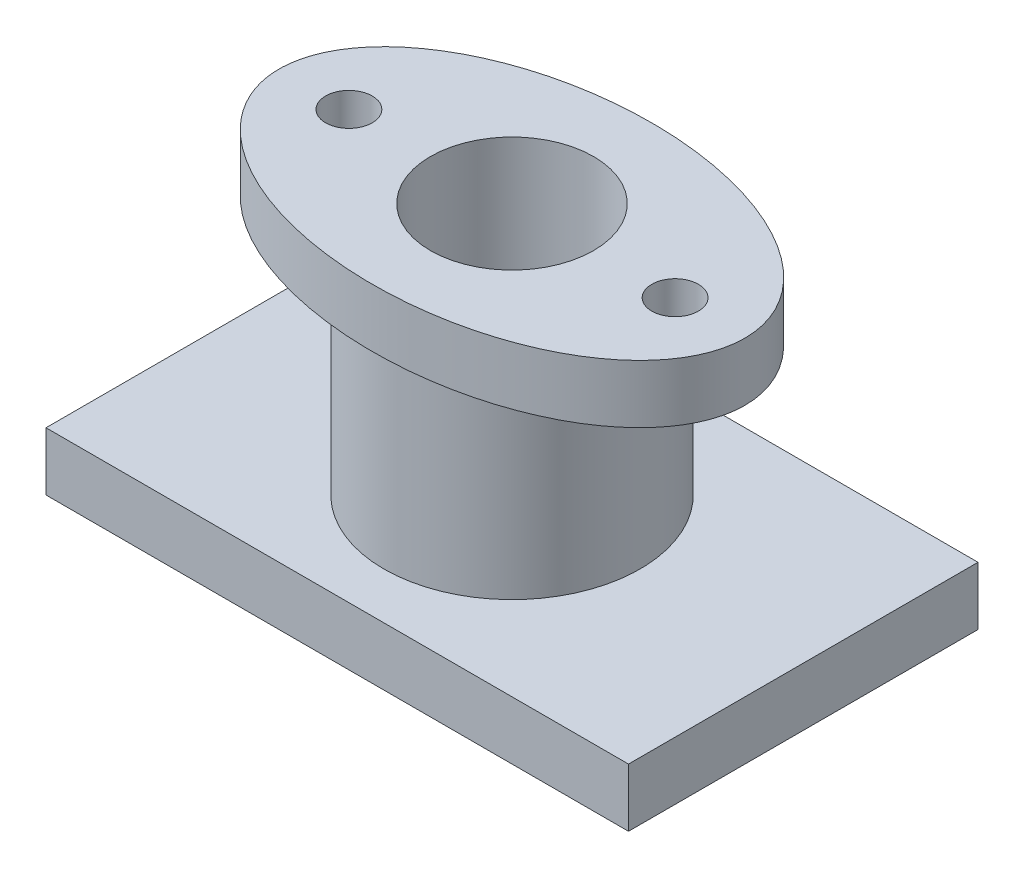
from build123d import *

# Parameters (mm, degrees)
BASE_PLATE_SKETCH_W        = 150
BASE_PLATE_SKETCH_H        = 90
BASE_PLATE_150X90X15_DEPTH = 15
BOSS_TUBE_SKETCH_R         = 33
BOSS_TUBE_SKETCH_R_2       = 21
BOSS_TUBE_66_DEPTH         = 50
OVAL_FLANGE_SKETCH_RX      = 60
OVAL_FLANGE_SKETCH_RY      = 36
OVAL_FLANGE_SKETCH_R       = 21
OVAL_FLANGE_120X72_DEPTH   = 15
BASE_BORE_SKETCH_R         = 16.5
BASE_BORE_33_DEPTH         = 15
FLANGE_BOLT_HOLE_SKETCH_R  = 6
FLANGE_BOLT_HOLE_DEPTH     = 15


with BuildPart() as part:
    # Base Plate Sketch → Base Plate 150x90x15 (new body)
    with BuildSketch(Plane(origin=(0, 0, 0), x_dir=(1, 0, 0), z_dir=(0, 1, 0))):
        Rectangle(BASE_PLATE_SKETCH_W, BASE_PLATE_SKETCH_H)
    extrude(amount=BASE_PLATE_150X90X15_DEPTH)

    # Boss Tube Sketch → Boss Tube Ø66 (add)
    with BuildSketch(Plane(origin=(0, 15, 0), x_dir=(1, 0, 0), z_dir=(0, 1, 0))):
        with Locations(Location((0, 0, 0), (0, 0, 90))):
            Circle(BOSS_TUBE_SKETCH_R)
        with Locations(Location((0, 0, 0), (0, 0, 270))):
            Circle(BOSS_TUBE_SKETCH_R_2, mode=Mode.SUBTRACT)
    extrude(amount=BOSS_TUBE_66_DEPTH)

    # Oval Flange Sketch → Oval Flange 120x72 (add)
    with BuildSketch(Plane(origin=(0, 65, 0), x_dir=(1, 0, 0), z_dir=(0, 1, 0))):
        with Locations((0, 0)):
            Ellipse(OVAL_FLANGE_SKETCH_RX, OVAL_FLANGE_SKETCH_RY)
        with Locations(Location((0, 0, 0), (0, 0, 270))):
            Circle(OVAL_FLANGE_SKETCH_R, mode=Mode.SUBTRACT)
    extrude(amount=OVAL_FLANGE_120X72_DEPTH)

    # Base Bore Sketch → Base Bore Ø33 (cut)
    with BuildSketch(Plane(origin=(0, 15, 0), x_dir=(1, 0, 0), z_dir=(0, 1, 0))):
        with Locations(Location((0, 0, 0), (0, 0, 270))):
            Circle(BASE_BORE_SKETCH_R)
    extrude(amount=-BASE_BORE_33_DEPTH, mode=Mode.SUBTRACT)

    # Flange Bolt Hole Sketch → Flange Bolt Hole (cut)
    with BuildSketch(Plane(origin=(0, 80, 0), x_dir=(1, 0, 0), z_dir=(0, 1, 0))):
        with Locations(Location((-41.995846121, 0, 0), (0, 0, 270))):
            Circle(FLANGE_BOLT_HOLE_SKETCH_R)
        with Locations(Location((41.995846121, 0, 0), (0, 0, 90))):
            Circle(FLANGE_BOLT_HOLE_SKETCH_R)
    extrude(amount=-FLANGE_BOLT_HOLE_DEPTH, mode=Mode.SUBTRACT)


solid = part.part
